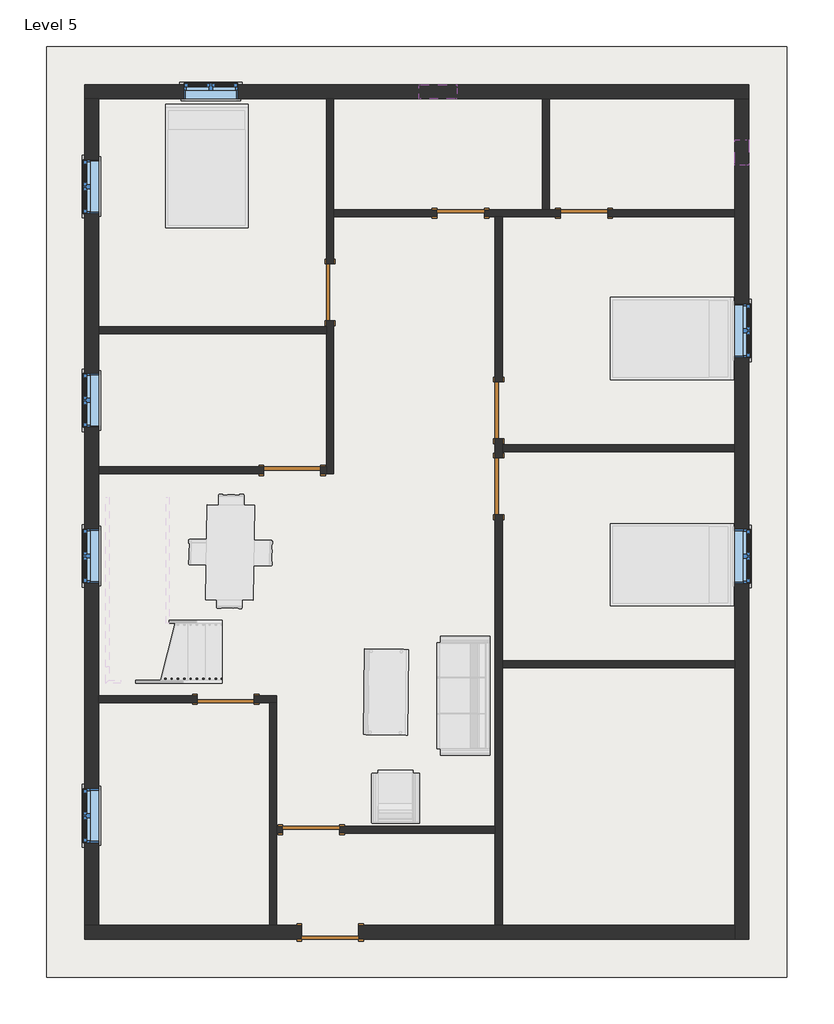
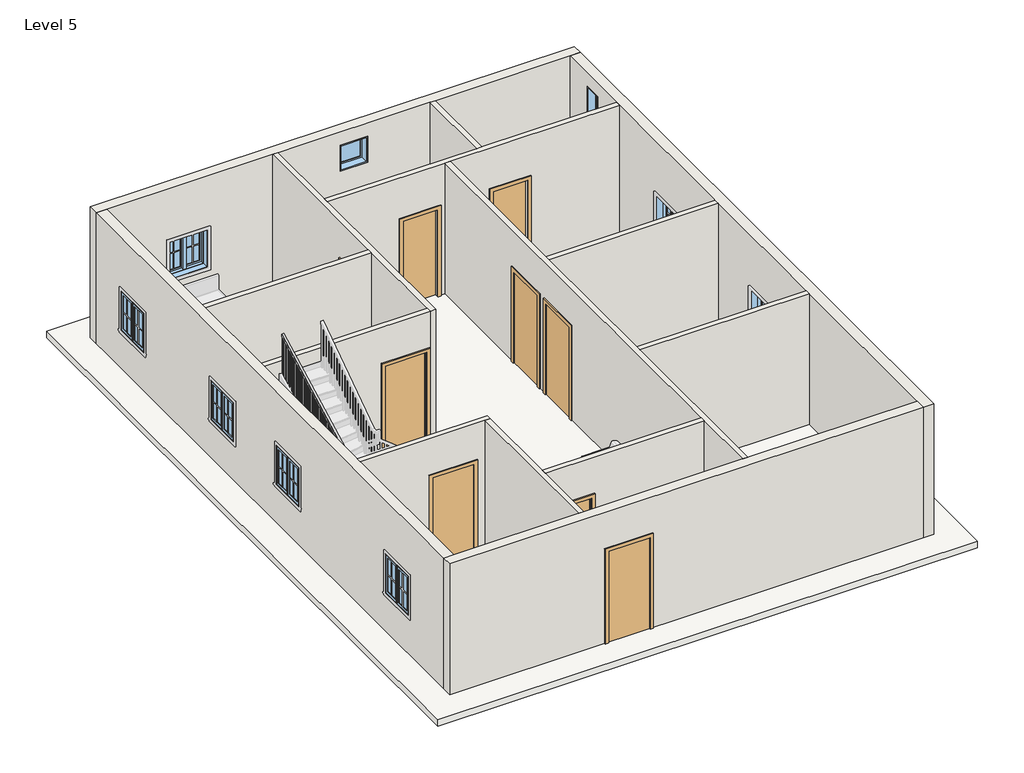
# One storey, part 1 of 2: 15 walls, 9 doors, 9 windows, 1 railing, 1 roof.
"""IFC4 building model written with IfcOpenShell, lengths in millimetres."""

from ifc_helpers import new_model, si_unit, frame, origin, place, context, project, spatial, polyline, outline, extrude, faceted_brep, transform, mapped, element, save
from components import door_d8f5dbb5, door_f2b275c1, door_305aa2a5, door_e5f9f3c4, door_0ca8825f, window_aa618e30, window_80340324, window_339605e1

model = new_model("IFC4")

# Units and contexts
model_context = context("Model", 3, world=origin())
ifc_project = project(units=[si_unit("LENGTHUNIT", "METRE", prefix="MILLI")], contexts=[model_context])

# Site, building, storey
site = spatial("IfcSite", under=ifc_project)
building = spatial("IfcBuilding", under=site)
storey = spatial("IfcBuildingStorey", under=building, Name="Level 5", Elevation=9601.2)

# Doors
placement = place(None, origin())
door_shape = door_d8f5dbb5(model_context)
element("IfcDoor", 1, ObjectType="Single-Flush : 30\" x 80\"", at=placement, inside=storey, context=model_context, shape_type="MappedRepresentation", body=[
    mapped(door_shape, transform((-551.6099931, 5332.4435985, 9601.2), x_axis=(1.0, 0.0, 0.0), y_axis=(0.0, 1.0, 0.0), z_axis=(0.0, 0.0, 1.0))),
])
door_2_shape = door_f2b275c1(model_context)
element("IfcDoor", 2, ObjectType="Single-Flush : 30\" x 80\"", at=placement, inside=storey, context=model_context, shape_type="MappedRepresentation", body=[
    mapped(door_2_shape, transform((1429.5900069, 5332.4435985, 9601.2), x_axis=(-1.0, 0.0, 0.0), y_axis=(0.0, -1.0, 0.0), z_axis=(0.0, 0.0, 1.0))),
])
door_3_shape = door_305aa2a5(model_context)
element("IfcDoor", 3, ObjectType="Single-Flush : 36\" x 84\"", at=placement, inside=storey, context=model_context, shape_type="MappedRepresentation", body=[
    mapped(door_3_shape, transform((-2647.1099931, 4062.4435985, 9601.2), x_axis=(0.0, -1.0, 0.0), y_axis=(1.0, 0.0, 0.0), z_axis=(0.0, 0.0, 1.0))),
])
element("IfcDoor", 4, ObjectType="Single-Flush : 36\" x 84\"", at=placement, inside=storey, context=model_context, shape_type="MappedRepresentation", body=[
    mapped(door_3_shape, transform((57.9900069, 2170.1435985, 9601.2), x_axis=(0.0, -1.0, 0.0), y_axis=(1.0, 0.0, 0.0), z_axis=(0.0, 0.0, 1.0))),
])
element("IfcDoor", 5, ObjectType="Single-Flush : 36\" x 84\"", at=placement, inside=storey, context=model_context, shape_type="MappedRepresentation", body=[
    mapped(door_3_shape, transform((-4323.5099931, -2465.3564015, 9601.2), x_axis=(1.0, 0.0, 0.0), y_axis=(0.0, 1.0, 0.0), z_axis=(0.0, 0.0, 1.0))),
])
element("IfcDoor", 6, ObjectType="Single-Flush : 36\" x 84\"", at=placement, inside=storey, context=model_context, shape_type="MappedRepresentation", body=[
    mapped(door_3_shape, transform((-2951.9099931, -4560.8564015, 9601.2), x_axis=(-1.0, 0.0, 0.0), y_axis=(0.0, -1.0, 0.0), z_axis=(0.0, 0.0, 1.0))),
])
door_4_shape = door_e5f9f3c4(model_context)
element("IfcDoor", 7, ObjectType="Single-Flush : 36\" x 84\"", at=placement, inside=storey, context=model_context, shape_type="MappedRepresentation", body=[
    mapped(door_4_shape, transform((-3256.7099931, 1204.9435985, 9601.2), x_axis=(1.0, 0.0, 0.0), y_axis=(0.0, 1.0, 0.0), z_axis=(0.0, 0.0, 1.0))),
])
element("IfcDoor", 8, ObjectType="Single-Flush : 36\" x 84\"", at=placement, inside=storey, context=model_context, shape_type="MappedRepresentation", body=[
    mapped(door_4_shape, transform((57.9900069, 950.9435985, 9601.2), x_axis=(0.0, 1.0, 0.0), y_axis=(-1.0, 0.0, 0.0), z_axis=(0.0, 0.0, 1.0))),
])
door_5_shape = door_0ca8825f(model_context)
element("IfcDoor", 9, ObjectType="Single-Flush : 36\" x 84\"", at=placement, inside=storey, context=model_context, shape_type="MappedRepresentation", body=[
    mapped(door_5_shape, transform((-2647.1099931, -6205.5064015, 9601.2), x_axis=(-1.0, 0.0, 0.0), y_axis=(0.0, -1.0, 0.0), z_axis=(0.0, 0.0, 1.0))),
])

# Railing
element("IfcRailing", 10, ObjectType="Handrail - Rectangular", at=placement, inside=storey, context=model_context, shape_type="SolidModel", body=[
    faceted_brep([(-4378.4230036, -2160.5564015, 11362.2666667), (-4378.4230036, -2160.5564015, 11306.1107192), (-4378.4230036, -2109.7564015, 11306.1107192), (-4378.4230036, -2109.7564015, 11362.2666667), (-5973.5005957, -2160.5564015, 12113.7835228), (-5984.8684735, -2160.5564015, 12062.9835228), (-5984.8684735, -2109.7564015, 12062.9835228), (-5973.5005957, -2109.7564015, 12113.7835228), (-6196.7599931, -2160.5564015, 12113.7835228), (-6196.7599931, -2160.5564015, 12062.9835228), (-6145.9599931, -2109.7564015, 12062.9835228), (-6145.9599931, -2109.7564015, 12113.7835228), (-6196.7599931, -1959.3194067, 12113.7835228), (-6196.7599931, -1946.6862419, 12062.9835228), (-6145.9599931, -1946.6862419, 12062.9835228), (-6145.9599931, -1959.3194067, 12113.7835228), (-6196.7599931, 775.380588, 13563.6), (-6145.9599931, 775.380588, 13563.6), (-6145.9599931, 775.380588, 13506.1024571), (-6196.7599931, 775.380588, 13506.1024571)], [[[0, 1, 2, 3]], [[1, 0, 4, 5]], [[2, 1, 5, 6]], [[3, 2, 6, 7]], [[0, 3, 7, 4]], [[5, 4, 8, 9]], [[6, 5, 9, 10]], [[7, 6, 10, 11]], [[4, 7, 11, 8]], [[9, 8, 12, 13]], [[10, 9, 13, 14]], [[11, 10, 14, 15]], [[8, 11, 15, 12]], [[16, 17, 18, 19]], [[13, 12, 16, 19]], [[14, 13, 19, 18]], [[15, 14, 18, 17]], [[12, 15, 17, 16]]]),
    extrude(outline(polyline([(719.1685985, 13476.3013569), (719.1685985, 12479.8666667), (700.1185985, 12479.8666667), (700.1185985, 13466.201893), (719.1685985, 13476.3013569)])), frame((-6180.8849931, 0.0, 0.0), z_axis=(1.0, 0.0, 0.0), x_axis=(0.0, 1.0, 0.0)), (0.0, 0.0, 1.0), 19.05),
    extrude(outline(polyline([(617.5685985, 13422.4375494), (617.5685985, 12479.8666667), (598.5185985, 12479.8666667), (598.5185985, 13412.3380855), (617.5685985, 13422.4375494)])), frame((-6180.8849931, 0.0, 0.0), z_axis=(1.0, 0.0, 0.0), x_axis=(0.0, 1.0, 0.0)), (0.0, 0.0, 1.0), 19.05),
    extrude(outline(polyline([(515.9685985, 13368.5737419), (515.9685985, 12479.8666667), (496.9185985, 12479.8666667), (496.9185985, 13358.474278), (515.9685985, 13368.5737419)])), frame((-6180.8849931, 0.0, 0.0), z_axis=(1.0, 0.0, 0.0), x_axis=(0.0, 1.0, 0.0)), (0.0, 0.0, 1.0), 19.05),
    extrude(outline(polyline([(414.3685985, 13314.7099344), (414.3685985, 12310.5333333), (395.3185985, 12310.5333333), (395.3185985, 13304.6104705), (414.3685985, 13314.7099344)])), frame((-6180.8849931, 0.0, 0.0), z_axis=(1.0, 0.0, 0.0), x_axis=(0.0, 1.0, 0.0)), (0.0, 0.0, 1.0), 19.05),
    extrude(outline(polyline([(312.7685985, 13260.8461269), (312.7685985, 12310.5333333), (293.7185985, 12310.5333333), (293.7185985, 13250.746663), (312.7685985, 13260.8461269)])), frame((-6180.8849931, 0.0, 0.0), z_axis=(1.0, 0.0, 0.0), x_axis=(0.0, 1.0, 0.0)), (0.0, 0.0, 1.0), 19.05),
    extrude(outline(polyline([(211.1685985, 13206.9823194), (211.1685985, 12141.2), (192.1185985, 12141.2), (192.1185985, 13196.8828555), (211.1685985, 13206.9823194)])), frame((-6180.8849931, 0.0, 0.0), z_axis=(1.0, 0.0, 0.0), x_axis=(0.0, 1.0, 0.0)), (0.0, 0.0, 1.0), 19.05),
    extrude(outline(polyline([(109.5685985, 13153.1185119), (109.5685985, 12141.2), (90.5185985, 12141.2), (90.5185985, 13143.019048), (109.5685985, 13153.1185119)])), frame((-6180.8849931, 0.0, 0.0), z_axis=(1.0, 0.0, 0.0), x_axis=(0.0, 1.0, 0.0)), (0.0, 0.0, 1.0), 19.05),
    extrude(outline(polyline([(7.9685985, 13099.2547044), (7.9685985, 12141.2), (-11.0814015, 12141.2), (-11.0814015, 13089.1552405), (7.9685985, 13099.2547044)])), frame((-6180.8849931, 0.0, 0.0), z_axis=(1.0, 0.0, 0.0), x_axis=(0.0, 1.0, 0.0)), (0.0, 0.0, 1.0), 19.05),
    extrude(outline(polyline([(-93.6314015, 13045.3908969), (-93.6314015, 11971.8666667), (-112.6814015, 11971.8666667), (-112.6814015, 13035.291433), (-93.6314015, 13045.3908969)])), frame((-6180.8849931, 0.0, 0.0), z_axis=(1.0, 0.0, 0.0), x_axis=(0.0, 1.0, 0.0)), (0.0, 0.0, 1.0), 19.05),
    extrude(outline(polyline([(-195.2314015, 12991.5270894), (-195.2314015, 11971.8666667), (-214.2814015, 11971.8666667), (-214.2814015, 12981.4276255), (-195.2314015, 12991.5270894)])), frame((-6180.8849931, 0.0, 0.0), z_axis=(1.0, 0.0, 0.0), x_axis=(0.0, 1.0, 0.0)), (0.0, 0.0, 1.0), 19.05),
    extrude(outline(polyline([(-296.8314015, 12937.6632819), (-296.8314015, 11971.8666667), (-315.8814015, 11971.8666667), (-315.8814015, 12927.563818), (-296.8314015, 12937.6632819)])), frame((-6180.8849931, 0.0, 0.0), z_axis=(1.0, 0.0, 0.0), x_axis=(0.0, 1.0, 0.0)), (0.0, 0.0, 1.0), 19.05),
    extrude(outline(polyline([(-398.4314015, 12883.7994744), (-398.4314015, 11802.5333333), (-417.4814015, 11802.5333333), (-417.4814015, 12873.7000105), (-398.4314015, 12883.7994744)])), frame((-6180.8849931, 0.0, 0.0), z_axis=(1.0, 0.0, 0.0), x_axis=(0.0, 1.0, 0.0)), (0.0, 0.0, 1.0), 19.05),
    extrude(outline(polyline([(-500.0314015, 12829.9356669), (-500.0314015, 11802.5333333), (-519.0814015, 11802.5333333), (-519.0814015, 12819.836203), (-500.0314015, 12829.9356669)])), frame((-6180.8849931, 0.0, 0.0), z_axis=(1.0, 0.0, 0.0), x_axis=(0.0, 1.0, 0.0)), (0.0, 0.0, 1.0), 19.05),
    extrude(outline(polyline([(-601.6314015, 12776.0718594), (-601.6314015, 11802.5333333), (-620.6814015, 11802.5333333), (-620.6814015, 12765.9723955), (-601.6314015, 12776.0718594)])), frame((-6180.8849931, 0.0, 0.0), z_axis=(1.0, 0.0, 0.0), x_axis=(0.0, 1.0, 0.0)), (0.0, 0.0, 1.0), 19.05),
    extrude(outline(polyline([(-703.2314015, 12722.2080519), (-703.2314015, 11633.2), (-722.2814015, 11633.2), (-722.2814015, 12712.108588), (-703.2314015, 12722.2080519)])), frame((-6180.8849931, 0.0, 0.0), z_axis=(1.0, 0.0, 0.0), x_axis=(0.0, 1.0, 0.0)), (0.0, 0.0, 1.0), 19.05),
    extrude(outline(polyline([(-804.8314015, 12668.3442444), (-804.8314015, 11633.2), (-823.8814015, 11633.2), (-823.8814015, 12658.2447805), (-804.8314015, 12668.3442444)])), frame((-6180.8849931, 0.0, 0.0), z_axis=(1.0, 0.0, 0.0), x_axis=(0.0, 1.0, 0.0)), (0.0, 0.0, 1.0), 19.05),
    extrude(outline(polyline([(-906.4314015, 12614.4804369), (-906.4314015, 11633.2), (-925.4814015, 11633.2), (-925.4814015, 12604.380973), (-906.4314015, 12614.4804369)])), frame((-6180.8849931, 0.0, 0.0), z_axis=(1.0, 0.0, 0.0), x_axis=(0.0, 1.0, 0.0)), (0.0, 0.0, 1.0), 19.05),
    extrude(outline(polyline([(-1008.0314015, 12560.6166294), (-1008.0314015, 11463.8666667), (-1027.0814015, 11463.8666667), (-1027.0814015, 12550.5171655), (-1008.0314015, 12560.6166294)])), frame((-6180.8849931, 0.0, 0.0), z_axis=(1.0, 0.0, 0.0), x_axis=(0.0, 1.0, 0.0)), (0.0, 0.0, 1.0), 19.05),
    extrude(outline(polyline([(-1109.6314015, 12506.7528219), (-1109.6314015, 11463.8666667), (-1128.6814015, 11463.8666667), (-1128.6814015, 12496.653358), (-1109.6314015, 12506.7528219)])), frame((-6180.8849931, 0.0, 0.0), z_axis=(1.0, 0.0, 0.0), x_axis=(0.0, 1.0, 0.0)), (0.0, 0.0, 1.0), 19.05),
    extrude(outline(polyline([(-1211.2314015, 12452.8890144), (-1211.2314015, 11463.8666667), (-1230.2814015, 11463.8666667), (-1230.2814015, 12442.7895505), (-1211.2314015, 12452.8890144)])), frame((-6180.8849931, 0.0, 0.0), z_axis=(1.0, 0.0, 0.0), x_axis=(0.0, 1.0, 0.0)), (0.0, 0.0, 1.0), 19.05),
    extrude(outline(polyline([(-1312.8314015, 12399.0252069), (-1312.8314015, 11463.8666667), (-1331.8814015, 11463.8666667), (-1331.8814015, 12388.925743), (-1312.8314015, 12399.0252069)])), frame((-6180.8849931, 0.0, 0.0), z_axis=(1.0, 0.0, 0.0), x_axis=(0.0, 1.0, 0.0)), (0.0, 0.0, 1.0), 19.05),
    extrude(outline(polyline([(-1414.4314015, 12345.1613994), (-1414.4314015, 11294.5333333), (-1433.4814015, 11294.5333333), (-1433.4814015, 12335.0619355), (-1414.4314015, 12345.1613994)])), frame((-6180.8849931, 0.0, 0.0), z_axis=(1.0, 0.0, 0.0), x_axis=(0.0, 1.0, 0.0)), (0.0, 0.0, 1.0), 19.05),
    extrude(outline(polyline([(-1516.0314015, 12291.2975919), (-1516.0314015, 11294.5333333), (-1535.0814015, 11294.5333333), (-1535.0814015, 12281.198128), (-1516.0314015, 12291.2975919)])), frame((-6180.8849931, 0.0, 0.0), z_axis=(1.0, 0.0, 0.0), x_axis=(0.0, 1.0, 0.0)), (0.0, 0.0, 1.0), 19.05),
    extrude(outline(polyline([(-1617.6314015, 12237.4337844), (-1617.6314015, 11294.5333333), (-1636.6814015, 11294.5333333), (-1636.6814015, 12227.3343205), (-1617.6314015, 12237.4337844)])), frame((-6180.8849931, 0.0, 0.0), z_axis=(1.0, 0.0, 0.0), x_axis=(0.0, 1.0, 0.0)), (0.0, 0.0, 1.0), 19.05),
    extrude(outline(polyline([(-1719.2314015, 12183.5699769), (-1719.2314015, 11294.5333333), (-1738.2814015, 11294.5333333), (-1738.2814015, 12173.470513), (-1719.2314015, 12183.5699769)])), frame((-6180.8849931, 0.0, 0.0), z_axis=(1.0, 0.0, 0.0), x_axis=(0.0, 1.0, 0.0)), (0.0, 0.0, 1.0), 19.05),
    extrude(outline(polyline([(-1820.8314015, 12129.7061694), (-1820.8314015, 11125.2), (-1839.8814015, 11125.2), (-1839.8814015, 12119.6067055), (-1820.8314015, 12129.7061694)])), frame((-6180.8849931, 0.0, 0.0), z_axis=(1.0, 0.0, 0.0), x_axis=(0.0, 1.0, 0.0)), (0.0, 0.0, 1.0), 19.05),
    extrude(outline(polyline([(-1922.4314015, 12075.8423619), (-1922.4314015, 11125.2), (-1941.4814015, 11125.2), (-1941.4814015, 12065.742898), (-1922.4314015, 12075.8423619)])), frame((-6180.8849931, 0.0, 0.0), z_axis=(1.0, 0.0, 0.0), x_axis=(0.0, 1.0, 0.0)), (0.0, 0.0, 1.0), 19.05),
    extrude(outline(polyline([(-6180.8849931, -2043.0814015), (-6180.8849931, -2024.0314015), (-6161.8349931, -2024.0314015), (-6161.8349931, -2043.0814015), (-6180.8849931, -2043.0814015)])), frame((0.0, 0.0, 11125.2), z_axis=(0.0, 0.0, 1.0), x_axis=(1.0, 0.0, 0.0)), (0.0, 0.0, 1.0), 937.7835228),
    extrude(outline(polyline([(-6096.0980036, -2144.6814015), (-6115.1480036, -2144.6814015), (-6115.1480036, -2125.6314015), (-6096.0980036, -2125.6314015), (-6096.0980036, -2144.6814015)])), frame((0.0, 0.0, 11125.2), z_axis=(0.0, 0.0, 1.0), x_axis=(1.0, 0.0, 0.0)), (0.0, 0.0, 1.0), 937.7835228),
    extrude(outline(polyline([(-5994.4980036, -2144.6814015), (-6013.5480036, -2144.6814015), (-6013.5480036, -2125.6314015), (-5994.4980036, -2125.6314015), (-5994.4980036, -2144.6814015)])), frame((0.0, 0.0, 11125.2), z_axis=(0.0, 0.0, 1.0), x_axis=(1.0, 0.0, 0.0)), (0.0, 0.0, 1.0), 937.7835228),
    extrude(outline(polyline([(12028.627224, -5911.9480036), (11125.2, -5911.9480036), (11125.2, -5892.8980036), (12019.6518637, -5892.8980036), (12028.627224, -5911.9480036)])), frame((0.0, -2144.6814015, 0.0), z_axis=(0.0, 1.0, 0.0), x_axis=(0.0, 0.0, 1.0)), (0.0, 0.0, 1.0), 19.05),
    extrude(outline(polyline([(11980.7586357, -5810.3480036), (11125.2, -5810.3480036), (11125.2, -5791.2980036), (11971.7832754, -5791.2980036), (11980.7586357, -5810.3480036)])), frame((0.0, -2144.6814015, 0.0), z_axis=(0.0, 1.0, 0.0), x_axis=(0.0, 0.0, 1.0)), (0.0, 0.0, 1.0), 19.05),
    extrude(outline(polyline([(11932.8900474, -5708.7480036), (10955.8666667, -5708.7480036), (10955.8666667, -5689.6980036), (11923.9146871, -5689.6980036), (11932.8900474, -5708.7480036)])), frame((0.0, -2144.6814015, 0.0), z_axis=(0.0, 1.0, 0.0), x_axis=(0.0, 0.0, 1.0)), (0.0, 0.0, 1.0), 19.05),
    extrude(outline(polyline([(11885.0214591, -5607.1480036), (10955.8666667, -5607.1480036), (10955.8666667, -5588.0980036), (11876.0460988, -5588.0980036), (11885.0214591, -5607.1480036)])), frame((0.0, -2144.6814015, 0.0), z_axis=(0.0, 1.0, 0.0), x_axis=(0.0, 0.0, 1.0)), (0.0, 0.0, 1.0), 19.05),
    extrude(outline(polyline([(11837.1528708, -5505.5480036), (10955.8666667, -5505.5480036), (10955.8666667, -5486.4980036), (11828.1775105, -5486.4980036), (11837.1528708, -5505.5480036)])), frame((0.0, -2144.6814015, 0.0), z_axis=(0.0, 1.0, 0.0), x_axis=(0.0, 0.0, 1.0)), (0.0, 0.0, 1.0), 19.05),
    extrude(outline(polyline([(11789.2842825, -5403.9480036), (10955.8666667, -5403.9480036), (10955.8666667, -5384.8980036), (11780.3089222, -5384.8980036), (11789.2842825, -5403.9480036)])), frame((0.0, -2144.6814015, 0.0), z_axis=(0.0, 1.0, 0.0), x_axis=(0.0, 0.0, 1.0)), (0.0, 0.0, 1.0), 19.05),
    extrude(outline(polyline([(11741.4156942, -5302.3480036), (10786.5333333, -5302.3480036), (10786.5333333, -5283.2980036), (11732.4403338, -5283.2980036), (11741.4156942, -5302.3480036)])), frame((0.0, -2144.6814015, 0.0), z_axis=(0.0, 1.0, 0.0), x_axis=(0.0, 0.0, 1.0)), (0.0, 0.0, 1.0), 19.05),
    extrude(outline(polyline([(11693.5471058, -5200.7480036), (10786.5333333, -5200.7480036), (10786.5333333, -5181.6980036), (11684.5717455, -5181.6980036), (11693.5471058, -5200.7480036)])), frame((0.0, -2144.6814015, 0.0), z_axis=(0.0, 1.0, 0.0), x_axis=(0.0, 0.0, 1.0)), (0.0, 0.0, 1.0), 19.05),
    extrude(outline(polyline([(11645.6785175, -5099.1480036), (10786.5333333, -5099.1480036), (10786.5333333, -5080.0980036), (11636.7031572, -5080.0980036), (11645.6785175, -5099.1480036)])), frame((0.0, -2144.6814015, 0.0), z_axis=(0.0, 1.0, 0.0), x_axis=(0.0, 0.0, 1.0)), (0.0, 0.0, 1.0), 19.05),
    extrude(outline(polyline([(11597.8099292, -4997.5480036), (10786.5333333, -4997.5480036), (10786.5333333, -4978.4980036), (11588.8345689, -4978.4980036), (11597.8099292, -4997.5480036)])), frame((0.0, -2144.6814015, 0.0), z_axis=(0.0, 1.0, 0.0), x_axis=(0.0, 0.0, 1.0)), (0.0, 0.0, 1.0), 19.05),
    extrude(outline(polyline([(11549.9413409, -4895.9480036), (10617.2, -4895.9480036), (10617.2, -4876.8980036), (11540.9659806, -4876.8980036), (11549.9413409, -4895.9480036)])), frame((0.0, -2144.6814015, 0.0), z_axis=(0.0, 1.0, 0.0), x_axis=(0.0, 0.0, 1.0)), (0.0, 0.0, 1.0), 19.05),
    extrude(outline(polyline([(11502.0727526, -4794.3480036), (10617.2, -4794.3480036), (10617.2, -4775.2980036), (11493.0973923, -4775.2980036), (11502.0727526, -4794.3480036)])), frame((0.0, -2144.6814015, 0.0), z_axis=(0.0, 1.0, 0.0), x_axis=(0.0, 0.0, 1.0)), (0.0, 0.0, 1.0), 19.05),
    extrude(outline(polyline([(11454.2041643, -4692.7480036), (10617.2, -4692.7480036), (10617.2, -4673.6980036), (11445.228804, -4673.6980036), (11454.2041643, -4692.7480036)])), frame((0.0, -2144.6814015, 0.0), z_axis=(0.0, 1.0, 0.0), x_axis=(0.0, 0.0, 1.0)), (0.0, 0.0, 1.0), 19.05),
    extrude(outline(polyline([(11406.335576, -4591.1480036), (10447.8666667, -4591.1480036), (10447.8666667, -4572.0980036), (11397.3602157, -4572.0980036), (11406.335576, -4591.1480036)])), frame((0.0, -2144.6814015, 0.0), z_axis=(0.0, 1.0, 0.0), x_axis=(0.0, 0.0, 1.0)), (0.0, 0.0, 1.0), 19.05),
    extrude(outline(polyline([(11358.4669877, -4489.5480036), (10447.8666667, -4489.5480036), (10447.8666667, -4470.4980036), (11349.4916273, -4470.4980036), (11358.4669877, -4489.5480036)])), frame((0.0, -2144.6814015, 0.0), z_axis=(0.0, 1.0, 0.0), x_axis=(0.0, 0.0, 1.0)), (0.0, 0.0, 1.0), 19.05),
    extrude(outline(polyline([(-6161.8349931, -2144.6814015), (-6180.8849931, -2144.6814015), (-6180.8849931, -2125.6314015), (-6161.8349931, -2125.6314015), (-6161.8349931, -2144.6814015)])), frame((0.0, 0.0, 11125.2), z_axis=(0.0, 0.0, 1.0), x_axis=(1.0, 0.0, 0.0)), (0.0, 0.0, 1.0), 937.7835228),
    extrude(outline(polyline([(775.380588, 13506.1024571), (775.380588, 12479.8666667), (756.330588, 12479.8666667), (756.330588, 13496.0029932), (775.380588, 13506.1024571)])), frame((-6180.8849931, 0.0, 0.0), z_axis=(1.0, 0.0, 0.0), x_axis=(0.0, 1.0, 0.0)), (0.0, 0.0, 1.0), 19.05),
    extrude(outline(polyline([(11315.0860795, -4397.4730036), (10447.8666667, -4397.4730036), (10447.8666667, -4378.4230036), (11306.1107192, -4378.4230036), (11315.0860795, -4397.4730036)])), frame((0.0, -2144.6814015, 0.0), z_axis=(0.0, 1.0, 0.0), x_axis=(0.0, 0.0, 1.0)), (0.0, 0.0, 1.0), 19.05),
])

# Roof
element("IfcRoof", 11, ObjectType="Generic - 12\"", at=placement, inside=storey, context=model_context, shape_type="SweptSolid", body=[
    extrude(outline(polyline([(-7200.0599931, 8005.7935985), (4687.1400069, 8005.7935985), (4687.1400069, -6929.4064015), (-7200.0599931, -6929.4064015), (-7200.0599931, 8005.7935985)])), frame((0.0, 0.0, 9448.8), z_axis=(0.0, 0.0, 1.0), x_axis=(1.0, 0.0, 0.0)), (0.0, 0.0, 1.0), 152.4),
])

# Walls
element("IfcWall", 12, ObjectType="WALL4.5\"", at=placement, inside=storey, context=model_context, shape_type="SweptSolid", body=[
    extrude(outline(polyline([(-2704.2599931, 3395.6935985), (-6361.8599931, 3395.6935985), (-6361.8599931, 3509.9935985), (-2704.2599931, 3509.9935985), (-2704.2599931, 3395.6935985)])), frame((0.0, 0.0, 9601.2), z_axis=(0.0, 0.0, 1.0), x_axis=(1.0, 0.0, 0.0)), (0.0, 0.0, 1.0), 3048.0),
])
element("IfcWall", 13, ObjectType="WALL4.5\"", at=placement, inside=storey, context=model_context, shape_type="Brep", body=[
    faceted_brep([(-2704.2599931, 3605.2435985, 11734.8), (-2704.2599931, 3605.2435985, 9601.2), (-2704.2599931, 3509.9935985, 9601.2), (-2704.2599931, 3395.6935985, 9601.2), (-2704.2599931, 1262.0935985, 9601.2), (-2704.2599931, 1147.7935985, 9601.2), (-2704.2599931, 1147.7935985, 12649.2), (-2704.2599931, 1262.0935985, 12649.2), (-2704.2599931, 3395.6935985, 12649.2), (-2704.2599931, 3509.9935985, 12649.2), (-2704.2599931, 7167.5935985, 12649.2), (-2704.2599931, 7167.5935985, 9601.2), (-2704.2599931, 4519.6435985, 9601.2), (-2704.2599931, 4519.6435985, 11734.8), (-2589.9599931, 1147.7935985, 9601.2), (-2589.9599931, 3605.2435985, 9601.2), (-2589.9599931, 3605.2435985, 11734.8), (-2589.9599931, 4519.6435985, 11734.8), (-2589.9599931, 4519.6435985, 9601.2), (-2589.9599931, 5275.2935985, 9601.2), (-2589.9599931, 5389.5935985, 9601.2), (-2589.9599931, 7167.5935985, 9601.2), (-2589.9599931, 7167.5935985, 12649.2), (-2589.9599931, 5389.5935985, 12649.2), (-2589.9599931, 5275.2935985, 12649.2), (-2589.9599931, 1147.7935985, 12649.2)], [[[0, 1, 2, 3, 4, 5, 6, 7, 8, 9, 10, 11, 12, 13]], [[14, 15, 16, 17, 18, 19, 20, 21, 22, 23, 24, 25]], [[12, 11, 21, 20, 19, 18]], [[5, 4, 3, 2, 1, 15, 14]], [[11, 10, 22, 21]], [[6, 5, 14, 25]], [[16, 15, 1, 0]], [[17, 16, 0, 13]], [[18, 17, 13, 12]], [[10, 9, 8, 7, 6, 25, 24, 23, 22]]]),
])
element("IfcWall", 14, ObjectType="WALL4.5\"", at=placement, inside=storey, context=model_context, shape_type="SweptSolid", body=[
    extrude(outline(polyline([(11734.8, -2799.5099931), (9601.2, -2799.5099931), (9601.2, -2704.2599931), (12649.2, -2704.2599931), (12649.2, -6361.8599931), (9601.2, -6361.8599931), (9601.2, -3713.9099931), (11734.8, -3713.9099931), (11734.8, -2799.5099931)])), frame((0.0, 1147.7935985, 0.0), z_axis=(0.0, 1.0, 0.0), x_axis=(0.0, 0.0, 1.0)), (0.0, 0.0, 1.0), 114.3),
])
element("IfcWall", 15, ObjectType="WALL4.5\"", at=placement, inside=storey, context=model_context, shape_type="Brep", body=[
    faceted_brep([(-170.6099931, 5275.2935985, 9601.2), (0.8400069, 5275.2935985, 9601.2), (115.1400069, 5275.2935985, 9601.2), (1048.5900069, 5275.2935985, 9601.2), (1048.5900069, 5275.2935985, 11633.2), (1810.5900069, 5275.2935985, 11633.2), (1810.5900069, 5275.2935985, 9601.2), (3848.9400069, 5275.2935985, 9601.2), (3848.9400069, 5275.2935985, 12649.2), (115.1400069, 5275.2935985, 12649.2), (0.8400069, 5275.2935985, 12649.2), (-2589.9599931, 5275.2935985, 12649.2), (-2589.9599931, 5275.2935985, 9601.2), (-932.6099931, 5275.2935985, 9601.2), (-932.6099931, 5275.2935985, 11633.2), (-170.6099931, 5275.2935985, 11633.2), (1048.5900069, 5389.5935985, 11633.2), (1048.5900069, 5389.5935985, 9601.2), (877.1400069, 5389.5935985, 9601.2), (762.8400069, 5389.5935985, 9601.2), (-170.6099931, 5389.5935985, 9601.2), (-170.6099931, 5389.5935985, 11633.2), (-932.6099931, 5389.5935985, 11633.2), (-932.6099931, 5389.5935985, 9601.2), (-2589.9599931, 5389.5935985, 9601.2), (-2589.9599931, 5389.5935985, 12649.2), (762.8400069, 5389.5935985, 12649.2), (877.1400069, 5389.5935985, 12649.2), (3848.9400069, 5389.5935985, 12649.2), (3848.9400069, 5389.5935985, 9601.2), (1810.5900069, 5389.5935985, 9601.2), (1810.5900069, 5389.5935985, 11633.2)], [[[0, 1, 2, 3, 4, 5, 6, 7, 8, 9, 10, 11, 12, 13, 14, 15]], [[16, 17, 18, 19, 20, 21, 22, 23, 24, 25, 26, 27, 28, 29, 30, 31]], [[13, 12, 24, 23]], [[30, 29, 7, 6]], [[20, 19, 18, 17, 3, 2, 1, 0]], [[8, 7, 29, 28]], [[12, 11, 25, 24]], [[21, 20, 0, 15]], [[22, 21, 15, 14]], [[23, 22, 14, 13]], [[4, 3, 17, 16]], [[5, 4, 16, 31]], [[6, 5, 31, 30]], [[11, 10, 9, 8, 28, 27, 26, 25]]]),
])
element("IfcWall", 16, ObjectType="WALL4.5\"", at=placement, inside=storey, context=model_context, shape_type="SweptSolid", body=[
    extrude(outline(polyline([(762.8400069, 5389.5935985), (762.8400069, 7167.5935985), (877.1400069, 7167.5935985), (877.1400069, 5389.5935985), (762.8400069, 5389.5935985)])), frame((0.0, 0.0, 9601.2), z_axis=(0.0, 0.0, 1.0), x_axis=(1.0, 0.0, 0.0)), (0.0, 0.0, 1.0), 3048.0),
])
element("IfcWall", 17, ObjectType="WALL4.5\"", at=placement, inside=storey, context=model_context, shape_type="Brep", body=[
    faceted_brep([(0.8400069, 1712.9435985, 9601.2), (0.8400069, 1408.1435985, 9601.2), (0.8400069, 1408.1435985, 11734.8), (0.8400069, 493.7435985, 11734.8), (0.8400069, 493.7435985, 9601.2), (0.8400069, -4503.7064015, 9601.2), (0.8400069, -4618.0064015, 9601.2), (0.8400069, -6091.2064015, 9601.2), (0.8400069, -6091.2064015, 12649.2), (0.8400069, -4618.0064015, 12649.2), (0.8400069, -4503.7064015, 12649.2), (0.8400069, 5275.2935985, 12649.2), (0.8400069, 5275.2935985, 9601.2), (0.8400069, 2627.3435985, 9601.2), (0.8400069, 2627.3435985, 11734.8), (0.8400069, 1712.9435985, 11734.8), (115.1400069, 1408.1435985, 11734.8), (115.1400069, 1408.1435985, 9601.2), (115.1400069, 1503.3935985, 9601.2), (115.1400069, 1617.6935985, 9601.2), (115.1400069, 1712.9435985, 9601.2), (115.1400069, 1712.9435985, 11734.8), (115.1400069, 2627.3435985, 11734.8), (115.1400069, 2627.3435985, 9601.2), (115.1400069, 5275.2935985, 9601.2), (115.1400069, 5275.2935985, 12649.2), (115.1400069, 1617.6935985, 12649.2), (115.1400069, 1503.3935985, 12649.2), (115.1400069, -1850.058017, 12649.2), (115.1400069, -1964.358017, 12649.2), (115.1400069, -6091.2064015, 12649.2), (115.1400069, -6091.2064015, 9601.2), (115.1400069, -1964.358017, 9601.2), (115.1400069, -1850.058017, 9601.2), (115.1400069, 493.7435985, 9601.2), (115.1400069, 493.7435985, 11734.8)], [[[0, 1, 2, 3, 4, 5, 6, 7, 8, 9, 10, 11, 12, 13, 14, 15]], [[16, 17, 18, 19, 20, 21, 22, 23, 24, 25, 26, 27, 28, 29, 30, 31, 32, 33, 34, 35]], [[13, 12, 24, 23]], [[34, 33, 32, 31, 7, 6, 5, 4]], [[20, 19, 18, 17, 1, 0]], [[8, 7, 31, 30]], [[12, 11, 25, 24]], [[21, 20, 0, 15]], [[22, 21, 15, 14]], [[23, 22, 14, 13]], [[2, 1, 17, 16]], [[3, 2, 16, 35]], [[4, 3, 35, 34]], [[11, 10, 9, 8, 30, 29, 28, 27, 26, 25]]]),
])
element("IfcWall", 18, ObjectType="WALL4.5\"", at=placement, inside=storey, context=model_context, shape_type="SweptSolid", body=[
    extrude(outline(polyline([(3848.9400069, -1964.358017), (115.1400069, -1964.358017), (115.1400069, -1850.058017), (3848.9400069, -1850.058017), (3848.9400069, -1964.358017)])), frame((0.0, 0.0, 9601.2), z_axis=(0.0, 0.0, 1.0), x_axis=(1.0, 0.0, 0.0)), (0.0, 0.0, 1.0), 3048.0),
])
element("IfcWall", 19, ObjectType="WALL4.5\"", at=placement, inside=storey, context=model_context, shape_type="SweptSolid", body=[
    extrude(outline(polyline([(3848.9400069, 1503.3935985), (115.1400069, 1503.3935985), (115.1400069, 1617.6935985), (3848.9400069, 1617.6935985), (3848.9400069, 1503.3935985)])), frame((0.0, 0.0, 9601.2), z_axis=(0.0, 0.0, 1.0), x_axis=(1.0, 0.0, 0.0)), (0.0, 0.0, 1.0), 3048.0),
])
element("IfcWall", 20, ObjectType="WALL4.5\"", at=placement, inside=storey, context=model_context, shape_type="Brep", body=[
    faceted_brep([(-3866.3099931, -2522.5064015, 11734.8), (-3866.3099931, -2522.5064015, 9601.2), (-3618.6599931, -2522.5064015, 9601.2), (-3504.3599931, -2522.5064015, 9601.2), (-3504.3599931, -2522.5064015, 12649.2), (-3618.6599931, -2522.5064015, 12649.2), (-6361.8599931, -2522.5064015, 12649.2), (-6361.8599931, -2522.5064015, 9601.2), (-4780.7099931, -2522.5064015, 9601.2), (-4780.7099931, -2522.5064015, 11734.8), (-3504.3599931, -2408.2064015, 9601.2), (-3866.3099931, -2408.2064015, 9601.2), (-3866.3099931, -2408.2064015, 11734.8), (-4780.7099931, -2408.2064015, 11734.8), (-4780.7099931, -2408.2064015, 9601.2), (-6361.8599931, -2408.2064015, 9601.2), (-6361.8599931, -2408.2064015, 12649.2), (-3504.3599931, -2408.2064015, 12649.2)], [[[0, 1, 2, 3, 4, 5, 6, 7, 8, 9]], [[10, 11, 12, 13, 14, 15, 16, 17]], [[8, 7, 15, 14]], [[3, 2, 1, 11, 10]], [[7, 6, 16, 15]], [[4, 3, 10, 17]], [[12, 11, 1, 0]], [[13, 12, 0, 9]], [[14, 13, 9, 8]], [[6, 5, 4, 17, 16]]]),
])
element("IfcWall", 21, ObjectType="WALL4.5\"", at=placement, inside=storey, context=model_context, shape_type="SweptSolid", body=[
    extrude(outline(polyline([(9601.2, -3504.3599931), (9601.2, -3409.1099931), (11734.8, -3409.1099931), (11734.8, -2494.7099931), (9601.2, -2494.7099931), (9601.2, 0.8400069), (12649.2, 0.8400069), (12649.2, -3504.3599931), (9601.2, -3504.3599931)])), frame((0.0, -4618.0064015, 0.0), z_axis=(0.0, 1.0, 0.0), x_axis=(0.0, 0.0, 1.0)), (0.0, 0.0, 1.0), 114.3),
])
element("IfcWall", 22, ObjectType="WALL4.5\"", at=placement, inside=storey, context=model_context, shape_type="Brep", body=[
    faceted_brep([(-3504.3599931, -6091.2064015, 9601.2), (-3504.3599931, -4618.0064015, 9601.2), (-3504.3599931, -4503.7064015, 9601.2), (-3504.3599931, -2522.5064015, 9601.2), (-3504.3599931, -2522.5064015, 12649.2), (-3504.3599931, -4503.7064015, 12649.2), (-3504.3599931, -4618.0064015, 12649.2), (-3504.3599931, -6091.2064015, 12649.2), (-3618.6599931, -6091.2064015, 9601.2), (-3618.6599931, -6091.2064015, 12649.2), (-3618.6599931, -2522.5064015, 12649.2), (-3618.6599931, -2522.5064015, 9601.2)], [[[0, 1, 2, 3, 4, 5, 6, 7]], [[8, 9, 10, 11]], [[3, 2, 1, 0, 8, 11]], [[4, 3, 11, 10]], [[0, 7, 9, 8]], [[7, 6, 5, 4, 10, 9]]]),
])
element("IfcWall", 23, ObjectType="WALL9\"", at=placement, inside=storey, context=model_context, shape_type="Brep", body=[
    faceted_brep([(-6590.4599931, 7167.5935985, 9601.2), (-6361.8599931, 7167.5935985, 9601.2), (-2704.2599931, 7167.5935985, 9601.2), (-2589.9599931, 7167.5935985, 9601.2), (762.8400069, 7167.5935985, 9601.2), (877.1400069, 7167.5935985, 9601.2), (3848.9400069, 7167.5935985, 9601.2), (4077.5400069, 7167.5935985, 9601.2), (4077.5400069, 7167.5935985, 12649.2), (3848.9400069, 7167.5935985, 12649.2), (877.1400069, 7167.5935985, 12649.2), (762.8400069, 7167.5935985, 12649.2), (-2589.9599931, 7167.5935985, 12649.2), (-2704.2599931, 7167.5935985, 12649.2), (-6361.8599931, 7167.5935985, 12649.2), (-6590.4599931, 7167.5935985, 12649.2), (-608.7599931, 7167.5935985, 12344.4), (-608.7599931, 7167.5935985, 11734.8), (-1218.3599931, 7167.5935985, 11734.8), (-1218.3599931, 7167.5935985, 12344.4), (-4129.8349931, 7167.5935985, 11430.0), (-4129.8349931, 7167.5935985, 10515.6), (-4993.4349931, 7167.5935985, 10515.6), (-4993.4349931, 7167.5935985, 11430.0), (4077.5400069, 7396.1935985, 9601.2), (-6590.4599931, 7396.1935985, 9601.2), (-6590.4599931, 7396.1935985, 12649.2), (4077.5400069, 7396.1935985, 12649.2), (-608.7599931, 7396.1935985, 11734.8), (-608.7599931, 7396.1935985, 12344.4), (-1218.3599931, 7396.1935985, 12344.4), (-1218.3599931, 7396.1935985, 11734.8), (-4129.8349931, 7396.1935985, 10515.6), (-4129.8349931, 7396.1935985, 11430.0), (-4993.4349931, 7396.1935985, 11430.0), (-4993.4349931, 7396.1935985, 10515.6)], [[[0, 1, 2, 3, 4, 5, 6, 7, 8, 9, 10, 11, 12, 13, 14, 15], [16, 17, 18, 19], [20, 21, 22, 23]], [[24, 25, 26, 27], [28, 29, 30, 31], [32, 33, 34, 35]], [[7, 6, 5, 4, 3, 2, 1, 0, 25, 24]], [[8, 7, 24, 27]], [[0, 15, 26, 25]], [[16, 29, 28, 17]], [[17, 28, 31, 18]], [[18, 31, 30, 19]], [[21, 20, 33, 32]], [[22, 21, 32, 35]], [[23, 22, 35, 34]], [[20, 23, 34, 33]], [[15, 14, 13, 12, 11, 10, 9, 8, 27, 26]], [[29, 16, 19, 30]]]),
])
element("IfcWall", 24, ObjectType="WALL9\"", at=placement, inside=storey, context=model_context, shape_type="Brep", body=[
    faceted_brep([(3848.9400069, 7167.5935985, 9601.2), (3848.9400069, 5389.5935985, 9601.2), (3848.9400069, 5275.2935985, 9601.2), (3848.9400069, 1617.6935985, 9601.2), (3848.9400069, 1503.3935985, 9601.2), (3848.9400069, -1850.058017, 9601.2), (3848.9400069, -1964.358017, 9601.2), (3848.9400069, -6091.2064015, 9601.2), (3848.9400069, -6319.8064015, 9601.2), (3848.9400069, -6319.8064015, 12649.2), (3848.9400069, -6091.2064015, 12649.2), (3848.9400069, -1964.358017, 12649.2), (3848.9400069, -1850.058017, 12649.2), (3848.9400069, 1503.3935985, 12649.2), (3848.9400069, 1617.6935985, 12649.2), (3848.9400069, 5275.2935985, 12649.2), (3848.9400069, 5389.5935985, 12649.2), (3848.9400069, 7167.5935985, 12649.2), (3848.9400069, 6103.9685985, 12344.4), (3848.9400069, 6103.9685985, 11734.8), (3848.9400069, 6510.3685985, 11734.8), (3848.9400069, 6510.3685985, 12344.4), (3848.9400069, 3014.6935985, 11430.0), (3848.9400069, 3014.6935985, 10515.6), (3848.9400069, 3878.2935985, 10515.6), (3848.9400069, 3878.2935985, 11430.0), (3848.9400069, -605.1322092, 11430.0), (3848.9400069, -605.1322092, 10515.6), (3848.9400069, 258.4677908, 10515.6), (3848.9400069, 258.4677908, 11430.0), (4077.5400069, -6319.8064015, 9601.2), (4077.5400069, 7167.5935985, 9601.2), (4077.5400069, 7167.5935985, 12649.2), (4077.5400069, -6319.8064015, 12649.2), (4077.5400069, 6103.9685985, 11734.8), (4077.5400069, 6103.9685985, 12344.4), (4077.5400069, 6510.3685985, 12344.4), (4077.5400069, 6510.3685985, 11734.8), (4077.5400069, 3014.6935985, 10515.6), (4077.5400069, 3014.6935985, 11430.0), (4077.5400069, 3878.2935985, 11430.0), (4077.5400069, 3878.2935985, 10515.6), (4077.5400069, -605.1322092, 10515.6), (4077.5400069, -605.1322092, 11430.0), (4077.5400069, 258.4677908, 11430.0), (4077.5400069, 258.4677908, 10515.6)], [[[0, 1, 2, 3, 4, 5, 6, 7, 8, 9, 10, 11, 12, 13, 14, 15, 16, 17], [18, 19, 20, 21], [22, 23, 24, 25], [26, 27, 28, 29]], [[30, 31, 32, 33], [34, 35, 36, 37], [38, 39, 40, 41], [42, 43, 44, 45]], [[8, 7, 6, 5, 4, 3, 2, 1, 0, 31, 30]], [[0, 17, 32, 31]], [[9, 8, 30, 33]], [[18, 35, 34, 19]], [[19, 34, 37, 20]], [[20, 37, 36, 21]], [[23, 22, 39, 38]], [[24, 23, 38, 41]], [[25, 24, 41, 40]], [[22, 25, 40, 39]], [[27, 26, 43, 42]], [[28, 27, 42, 45]], [[29, 28, 45, 44]], [[26, 29, 44, 43]], [[17, 16, 15, 14, 13, 12, 11, 10, 9, 33, 32]], [[35, 18, 21, 36]]]),
])
element("IfcWall", 25, ObjectType="WALL9\"", at=placement, inside=storey, context=model_context, shape_type="Brep", body=[
    faceted_brep([(-3104.3099931, -6091.2064015, 11734.8), (-3104.3099931, -6091.2064015, 9601.2), (-3504.3599931, -6091.2064015, 9601.2), (-3618.6599931, -6091.2064015, 9601.2), (-6361.8599931, -6091.2064015, 9601.2), (-6590.4599931, -6091.2064015, 9601.2), (-6590.4599931, -6091.2064015, 12649.2), (-6361.8599931, -6091.2064015, 12649.2), (-3618.6599931, -6091.2064015, 12649.2), (-3504.3599931, -6091.2064015, 12649.2), (0.8400069, -6091.2064015, 12649.2), (115.1400069, -6091.2064015, 12649.2), (3848.9400069, -6091.2064015, 12649.2), (3848.9400069, -6091.2064015, 9601.2), (115.1400069, -6091.2064015, 9601.2), (0.8400069, -6091.2064015, 9601.2), (-2189.9099931, -6091.2064015, 9601.2), (-2189.9099931, -6091.2064015, 11734.8), (-6590.4599931, -6319.8064015, 9601.2), (-3104.3099931, -6319.8064015, 9601.2), (-3104.3099931, -6319.8064015, 11734.8), (-2189.9099931, -6319.8064015, 11734.8), (-2189.9099931, -6319.8064015, 9601.2), (3848.9400069, -6319.8064015, 9601.2), (3848.9400069, -6319.8064015, 12649.2), (-6590.4599931, -6319.8064015, 12649.2)], [[[0, 1, 2, 3, 4, 5, 6, 7, 8, 9, 10, 11, 12, 13, 14, 15, 16, 17]], [[18, 19, 20, 21, 22, 23, 24, 25]], [[5, 4, 3, 2, 1, 19, 18]], [[16, 15, 14, 13, 23, 22]], [[13, 12, 24, 23]], [[6, 5, 18, 25]], [[12, 11, 10, 9, 8, 7, 6, 25, 24]], [[20, 19, 1, 0]], [[21, 20, 0, 17]], [[22, 21, 17, 16]]]),
])
element("IfcWall", 26, ObjectType="WALL9\"", at=placement, inside=storey, context=model_context, shape_type="Brep", body=[
    faceted_brep([(-6361.8599931, -6091.2064015, 9601.2), (-6361.8599931, -2522.5064015, 9601.2), (-6361.8599931, -2408.2064015, 9601.2), (-6361.8599931, 1147.7935985, 9601.2), (-6361.8599931, 1262.0935985, 9601.2), (-6361.8599931, 3395.6935985, 9601.2), (-6361.8599931, 3509.9935985, 9601.2), (-6361.8599931, 7167.5935985, 9601.2), (-6361.8599931, 7167.5935985, 12649.2), (-6361.8599931, 3509.9935985, 12649.2), (-6361.8599931, 3395.6935985, 12649.2), (-6361.8599931, 1262.0935985, 12649.2), (-6361.8599931, 1147.7935985, 12649.2), (-6361.8599931, -2408.2064015, 12649.2), (-6361.8599931, -2522.5064015, 12649.2), (-6361.8599931, -6091.2064015, 12649.2), (-6361.8599931, 2760.6935985, 11430.0), (-6361.8599931, 2760.6935985, 10515.6), (-6361.8599931, 1897.0935985, 10515.6), (-6361.8599931, 1897.0935985, 11430.0), (-6361.8599931, 6189.6935985, 11430.0), (-6361.8599931, 6189.6935985, 10515.6), (-6361.8599931, 5326.0935985, 10515.6), (-6361.8599931, 5326.0935985, 11430.0), (-6361.8599931, -3903.6314015, 11430.0), (-6361.8599931, -3903.6314015, 10515.6), (-6361.8599931, -4767.2314015, 10515.6), (-6361.8599931, -4767.2314015, 11430.0), (-6361.8599931, 265.1435985, 11430.0), (-6361.8599931, 265.1435985, 10515.6), (-6361.8599931, -598.4564015, 10515.6), (-6361.8599931, -598.4564015, 11430.0), (-6590.4599931, -6091.2064015, 9601.2), (-6590.4599931, -6091.2064015, 12649.2), (-6590.4599931, 7167.5935985, 12649.2), (-6590.4599931, 7167.5935985, 9601.2), (-6590.4599931, 2760.6935985, 11430.0), (-6590.4599931, 1897.0935985, 11430.0), (-6590.4599931, 1897.0935985, 10515.6), (-6590.4599931, 2760.6935985, 10515.6), (-6590.4599931, 6189.6935985, 11430.0), (-6590.4599931, 5326.0935985, 11430.0), (-6590.4599931, 5326.0935985, 10515.6), (-6590.4599931, 6189.6935985, 10515.6), (-6590.4599931, -3903.6314015, 11430.0), (-6590.4599931, -4767.2314015, 11430.0), (-6590.4599931, -4767.2314015, 10515.6), (-6590.4599931, -3903.6314015, 10515.6), (-6590.4599931, 265.1435985, 11430.0), (-6590.4599931, -598.4564015, 11430.0), (-6590.4599931, -598.4564015, 10515.6), (-6590.4599931, 265.1435985, 10515.6)], [[[0, 1, 2, 3, 4, 5, 6, 7, 8, 9, 10, 11, 12, 13, 14, 15], [16, 17, 18, 19], [20, 21, 22, 23], [24, 25, 26, 27], [28, 29, 30, 31]], [[32, 33, 34, 35], [36, 37, 38, 39], [40, 41, 42, 43], [44, 45, 46, 47], [48, 49, 50, 51]], [[7, 6, 5, 4, 3, 2, 1, 0, 32, 35]], [[0, 15, 33, 32]], [[8, 7, 35, 34]], [[17, 16, 36, 39]], [[18, 17, 39, 38]], [[19, 18, 38, 37]], [[16, 19, 37, 36]], [[21, 20, 40, 43]], [[22, 21, 43, 42]], [[23, 22, 42, 41]], [[20, 23, 41, 40]], [[25, 24, 44, 47]], [[26, 25, 47, 46]], [[27, 26, 46, 45]], [[24, 27, 45, 44]], [[29, 28, 48, 51]], [[30, 29, 51, 50]], [[31, 30, 50, 49]], [[28, 31, 49, 48]], [[15, 14, 13, 12, 11, 10, 9, 8, 34, 33]]]),
])

# Windows
window_shape = window_aa618e30(model_context)
element("IfcWindow", 27, ObjectType="Fixed : 16\" x 24\"", at=placement, inside=storey, context=model_context, shape_type="MappedRepresentation", body=[
    mapped(window_shape, transform((3963.2400069, 6269.0685985, 10820.4), x_axis=(0.0, -1.0, 0.0), y_axis=(1.0, 0.0, 0.0), z_axis=(0.0, 0.0, 1.0))),
])
window_2_shape = window_80340324(model_context)
element("IfcWindow", 28, ObjectType="Fixed : 24\" x 24\"", at=placement, inside=storey, context=model_context, shape_type="MappedRepresentation", body=[
    mapped(window_2_shape, transform((-875.4599931, 7281.8935985, 10820.4), x_axis=(1.0, 0.0, 0.0), y_axis=(0.0, 1.0, 0.0), z_axis=(0.0, 0.0, 1.0))),
])
window_3_shape = window_339605e1(model_context)
element("IfcWindow", 29, ObjectType="Window-Casement-Double : 34\" x 36\"", at=placement, inside=storey, context=model_context, shape_type="MappedRepresentation", body=[
    mapped(window_3_shape, transform((-4561.6349931, 7281.8935985, 9601.2), x_axis=(1.0, 0.0, 0.0), y_axis=(0.0, 1.0, 0.0), z_axis=(0.0, 0.0, 1.0))),
])
element("IfcWindow", 30, ObjectType="Window-Casement-Double : 34\" x 36\"", at=placement, inside=storey, context=model_context, shape_type="MappedRepresentation", body=[
    mapped(window_3_shape, transform((3963.2400069, 3446.4935985, 9601.2), x_axis=(0.0, -1.0, 0.0), y_axis=(1.0, 0.0, 0.0), z_axis=(0.0, 0.0, 1.0))),
])
element("IfcWindow", 31, ObjectType="Window-Casement-Double : 34\" x 36\"", at=placement, inside=storey, context=model_context, shape_type="MappedRepresentation", body=[
    mapped(window_3_shape, transform((3963.2400069, -173.3322092, 9601.2), x_axis=(0.0, -1.0, 0.0), y_axis=(1.0, 0.0, 0.0), z_axis=(0.0, 0.0, 1.0))),
])
element("IfcWindow", 32, ObjectType="Window-Casement-Double : 34\" x 36\"", at=placement, inside=storey, context=model_context, shape_type="MappedRepresentation", body=[
    mapped(window_3_shape, transform((-6476.1599931, 2328.8935985, 9601.2), x_axis=(0.0, 1.0, 0.0), y_axis=(-1.0, 0.0, 0.0), z_axis=(0.0, 0.0, 1.0))),
])
element("IfcWindow", 33, ObjectType="Window-Casement-Double : 34\" x 36\"", at=placement, inside=storey, context=model_context, shape_type="MappedRepresentation", body=[
    mapped(window_3_shape, transform((-6476.1599931, 5757.8935985, 9601.2), x_axis=(0.0, 1.0, 0.0), y_axis=(-1.0, 0.0, 0.0), z_axis=(0.0, 0.0, 1.0))),
])
element("IfcWindow", 34, ObjectType="Window-Casement-Double : 34\" x 36\"", at=placement, inside=storey, context=model_context, shape_type="MappedRepresentation", body=[
    mapped(window_3_shape, transform((-6476.1599931, -4335.4314015, 9601.2), x_axis=(0.0, 1.0, 0.0), y_axis=(-1.0, 0.0, 0.0), z_axis=(0.0, 0.0, 1.0))),
])
element("IfcWindow", 35, ObjectType="Window-Casement-Double : 34\" x 36\"", at=placement, inside=storey, context=model_context, shape_type="MappedRepresentation", body=[
    mapped(window_3_shape, transform((-6476.1599931, -166.6564015, 9601.2), x_axis=(0.0, 1.0, 0.0), y_axis=(-1.0, 0.0, 0.0), z_axis=(0.0, 0.0, 1.0))),
])

save(model, "model.ifc")

# Revit data of these elements
# Type "Single-Flush : 30\" x 80\""
#   Type Mark = "5"
#   Construction Type Id = "MDOOR"
#   Assembly Code = "C1020"
#   Analytic Construction = "Metal"
#   Thickness = 0' - 2"
#   Heat Transfer Coefficient (U) = 0.651978 BTU/(h·ft²·°F)
#   Height = 6' - 8"
#   Trim Projection Ext = 0' - 1"
#   Trim Projection Int = 0' - 1"
#   Trim Width = 0' - 3"
#   Width = 2' - 6"
#   Define Thermal Properties by = 1
#   Define Thermal Properties by = 1
#   Door Material = Door - Panel
#   Frame Material = Door - Frame
#   Visual Light Transmittance = 0
#   Solar Heat Gain Coefficient = 0
#   Function = (empty or 0)
#   Wall Closure = (empty or 0)
# Type "Single-Flush : 36\" x 84\""
#   Type Mark = "1"
#   Construction Type Id = "MDOOR"
#   Assembly Code = "C1020"
#   Analytic Construction = "Metal"
#   Thickness = 0' - 2"
#   Heat Transfer Coefficient (U) = 0.651978 BTU/(h·ft²·°F)
#   Height = 7' - 0"
#   Trim Projection Ext = 0' - 1"
#   Trim Projection Int = 0' - 1"
#   Trim Width = 0' - 3"
#   Width = 3' - 0"
#   Define Thermal Properties by = 1
#   Define Thermal Properties by = 1
#   Door Material = Door - Panel
#   Frame Material = Door - Frame
#   Visual Light Transmittance = 0
#   Solar Heat Gain Coefficient = 0
#   Function = (empty or 0)
#   Wall Closure = (empty or 0)
# Type "Handrail - Rectangular"
#   Assembly Code = "C2010400"
#   built-in parameter 1008612 = 0.0416667 (stored number, unit not read)
#   built-in parameter 1008611 = 0.0416667 (stored number, unit not read)
#   built-in parameter 1008609 = 0.333333 (stored number, unit not read)
#   built-in parameter 1008604 = 0.166667 (stored number, unit not read)
#   built-in parameter 1008603 = 0.166667 (stored number, unit not read)
#   Railing Height = 3' - 0"
#   built-in parameter 1008630 = 2
#   built-in parameter 1008610 = 2
#   built-in parameter 1008618 = Baluster - Square : 3/4"
# Type "Generic - 12\""
#   Assembly Code = "B1020"
#   Layers, outside or top first: 0' - 6" no material (function 1)
# Type "WALL4.5\""
#   Assembly Code = "B2010"
#   Layers, outside or top first: 0' - 4 1/2" no material (function 1)
# Type "WALL9\""
#   Assembly Code = "B2010"
#   Layers, outside or top first: 0' - 9" no material (function 1)
# Type "Fixed : 16\" x 24\""
#   Type Mark = "4"
#   Construction Type Id = "GSP4R"
#   Assembly Code = "B2020100"
#   Analytic Construction = "1/8 in Pilkington single glazing"
#   Visual Light Transmittance = 0.9
#   Solar Heat Gain Coefficient = 0.78
#   Heat Transfer Coefficient (U) = 0.6496 BTU/(h·ft²·°F)
#   Height = 2' - 0"
#   Default Sill Height = 3' - 0"
#   Width = 1' - 4"
#   Window Inset = 0' - 0 3/4"
#   Define Thermal Properties by = 1
#   Define Thermal Properties by = 1
#   Glass Pane Material = Glass
#   Sash Material = Sash
#   Wall Closure = (empty or 0)
# Type "Fixed : 24\" x 24\""
#   Type Mark = "3"
#   Construction Type Id = "GSP4R"
#   Assembly Code = "B2020100"
#   Analytic Construction = "1/8 in Pilkington single glazing"
#   Visual Light Transmittance = 0.9
#   Solar Heat Gain Coefficient = 0.78
#   Heat Transfer Coefficient (U) = 0.6496 BTU/(h·ft²·°F)
#   Height = 2' - 0"
#   Default Sill Height = 3' - 0"
#   Width = 2' - 0"
#   Window Inset = 0' - 0 3/4"
#   Define Thermal Properties by = 1
#   Define Thermal Properties by = 1
#   Glass Pane Material = Glass
#   Sash Material = Sash
#   Wall Closure = (empty or 0)
# Type "Window-Casement-Double : 34\" x 36\""
#   Type Mark = "14"
#   Fire Rating = "0.5h"
#   Assembly Code = "B2020100"
#   Analytic Construction = "Double glazing - domestic"
#   Frame Extension [instance default] = 0' - 0 1/4"
#   Window Inset [instance default] = 0' - 0"
#   Wall Thickness [instance default] = 0' - 6"
#   Interior Wall Closure [instance default] = 0' - 2 1/4"
#   Half Width = 1' - 5"
#   Visual Light Transmittance = 0.81
#   Thermal Resistance (R) = 1.8146 (h·ft²·°F)/BTU
#   Solar Heat Gain Coefficient = 0.76
#   Rough Width = 2' - 10 1/2"
#   Rough Height = 3' - 0 1/2"
#   Height = 3' - 0"
#   Heat Transfer Coefficient (U) = 0.5511 BTU/(h·ft²·°F)
#   Exterior Wall Closure [instance default] = 0' - 1 1/4"
#   Extension Jamb [instance default] = 0' - 2 1/4"
#   Default Sill Height = 3' - 0"
#   Width = 2' - 10"
#   Define Thermal Properties by = 0
#   Muntin Visibility = yes
#   Interior Trim Visibility [instance default] = yes
#   Exterior Trim Visibility [instance default] = yes
#   Extension Jamb Visibility [instance default] = yes
#   Interior Trim Material = Wood - Stained
#   Muntin Pattern = Muntin Pattern_2x2 : Muntin Pattern_2x2
#   Interior Trim = Trim-Window-Interior-Flat : Picture Frame
#   Interior Frame Material = Wood - Stained
#   Glass Panel Material = Glass
#   Exterior Trim Material = Clad - White
#   Exterior Trim = Trim-Window-Exterior-Flat : with Sill
#   Exterior Frame Material = Clad - White
#   Wall Closure = (empty or 0)
# Elements 1, 2 (IfcDoor, "Single-Flush : 30\" x 80\"")
#   Phase Created = New Construction
#   Materials on its faces: "Door - Frame", "Door - Panel"
# Elements 3, 4, 5, 6, 7, 8, 9 (IfcDoor, "Single-Flush : 36\" x 84\"")
#   Phase Created = New Construction
#   Materials on its faces: "Door - Frame", "Door - Panel"
# Element 10 (IfcRailing, "Handrail - Rectangular")
#   Phase Created = New Construction
# Element 11 (IfcRoof, "Generic - 12\"")
#   built-in parameter 1001705 = 31.5 (stored number, unit not read)
#   built-in parameter 1001701 = -0.5 (stored number, unit not read)
#   built-in parameter 1001710 = 33615
#   Phase Created = New Construction
#   Materials on its faces: "Default Roof", "Oak Flooring"
# Elements 12, 13, 14, 15, 16, 17, 18, 19, 20, 21, 22 (IfcWall, "WALL4.5\"")
#   Top Offset = 0' - 0"
#   Base Offset = 0' - 0"
#   Unconnected Height = 10' - 0"
#   wall height = 10' - 0"
#   Phase Created = New Construction
#   Base Constraint = Level 5
#   Materials on its faces: "Default Wall"
# Elements 23, 24, 25, 26 (IfcWall, "WALL9\"")
#   Top Offset = 0' - 0"
#   Base Offset = 0' - 0"
#   Unconnected Height = 10' - 0"
#   wall height = 10' - 0"
#   Phase Created = New Construction
#   Base Constraint = Level 5
#   Materials on its faces: "Default Wall", "Oak Flooring"
# Element 27 (IfcWindow, "Fixed : 16\" x 24\"")
#   Mark = "29"
#   Phase Created = New Construction
#   Materials on its faces: "Sash", "Glass"
# Element 28 (IfcWindow, "Fixed : 24\" x 24\"")
#   Mark = "28"
#   Phase Created = New Construction
#   Materials on its faces: "Sash", "Glass"
# Element 29 (IfcWindow, "Window-Casement-Double : 34\" x 36\"")
#   Mark = "30"
#   Window Inset = 0' - 0"
#   Interior Wall Closure = 0' - 2 1/4"
#   Frame Extension = 0' - 0 1/4"
#   Exterior Wall Closure = 0' - 1 1/4"
#   Interior Trim Visibility = yes
#   Exterior Trim Visibility = yes
#   Phase Created = New Construction
#   Materials on its faces: "Wood - Stained", "Glass", "Clad - White"
# Element 30 (IfcWindow, "Window-Casement-Double : 34\" x 36\"")
#   Mark = "31"
#   Window Inset = 0' - 0"
#   Interior Wall Closure = 0' - 2 1/4"
#   Frame Extension = 0' - 0 1/4"
#   Exterior Wall Closure = 0' - 1 1/4"
#   Interior Trim Visibility = yes
#   Exterior Trim Visibility = yes
#   Phase Created = New Construction
#   Materials on its faces: "Wood - Stained", "Glass", "Clad - White"
# Element 31 (IfcWindow, "Window-Casement-Double : 34\" x 36\"")
#   Mark = "32"
#   Window Inset = 0' - 0"
#   Interior Wall Closure = 0' - 2 1/4"
#   Frame Extension = 0' - 0 1/4"
#   Exterior Wall Closure = 0' - 1 1/4"
#   Interior Trim Visibility = yes
#   Exterior Trim Visibility = yes
#   Phase Created = New Construction
#   Materials on its faces: "Wood - Stained", "Glass", "Clad - White"
# Element 32 (IfcWindow, "Window-Casement-Double : 34\" x 36\"")
#   Mark = "33"
#   Window Inset = 0' - 0"
#   Interior Wall Closure = 0' - 2 1/4"
#   Frame Extension = 0' - 0 1/4"
#   Exterior Wall Closure = 0' - 1 1/4"
#   Interior Trim Visibility = yes
#   Exterior Trim Visibility = yes
#   Phase Created = New Construction
#   Materials on its faces: "Wood - Stained", "Glass", "Clad - White"
# Element 33 (IfcWindow, "Window-Casement-Double : 34\" x 36\"")
#   Mark = "34"
#   Window Inset = 0' - 0"
#   Interior Wall Closure = 0' - 2 1/4"
#   Frame Extension = 0' - 0 1/4"
#   Exterior Wall Closure = 0' - 1 1/4"
#   Interior Trim Visibility = yes
#   Exterior Trim Visibility = yes
#   Phase Created = New Construction
#   Materials on its faces: "Wood - Stained", "Glass", "Clad - White"
# Element 34 (IfcWindow, "Window-Casement-Double : 34\" x 36\"")
#   Mark = "35"
#   Window Inset = 0' - 0"
#   Interior Wall Closure = 0' - 2 1/4"
#   Frame Extension = 0' - 0 1/4"
#   Exterior Wall Closure = 0' - 1 1/4"
#   Interior Trim Visibility = yes
#   Exterior Trim Visibility = yes
#   Phase Created = New Construction
#   Materials on its faces: "Wood - Stained", "Glass", "Clad - White"
# Element 35 (IfcWindow, "Window-Casement-Double : 34\" x 36\"")
#   Mark = "36"
#   Window Inset = 0' - 0"
#   Interior Wall Closure = 0' - 2 1/4"
#   Frame Extension = 0' - 0 1/4"
#   Exterior Wall Closure = 0' - 1 1/4"
#   Interior Trim Visibility = yes
#   Exterior Trim Visibility = yes
#   Phase Created = New Construction
#   Materials on its faces: "Wood - Stained", "Glass", "Clad - White"
# Materials
#   "Door - Panel": class "Wood", colour RGB 210 159 95, transparency 0, Cost = 0
#   "Door - Frame": colour RGB 118 70 51, transparency 0, Cost = 0
#   "Glass": class "Glass", colour RGB 0 128 192, transparency 0.75, Description = "Soda Lime Glass", Cost = 0
#   "Sash": class "Wood", colour RGB 224 178 126, transparency 0, Cost = 0
#   "Wood - Stained": class "Wood", colour RGB 224 178 126, transparency 0, Cost = 0
#   "Clad - White": class "Wood", colour RGB 242 242 238, transparency 0, Cost = 0
#   "Default Roof": colour RGB 88 101 114, transparency 0, Cost = 0
#   "Oak Flooring": class "Wood", colour RGB 216 169 114, transparency 0, Description = "Quercus Rubra", Cost = 0
#   "Default Wall": colour RGB 128 128 128, transparency 0, Cost = 0
